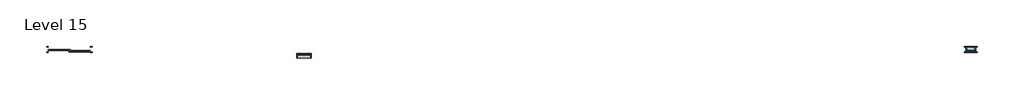
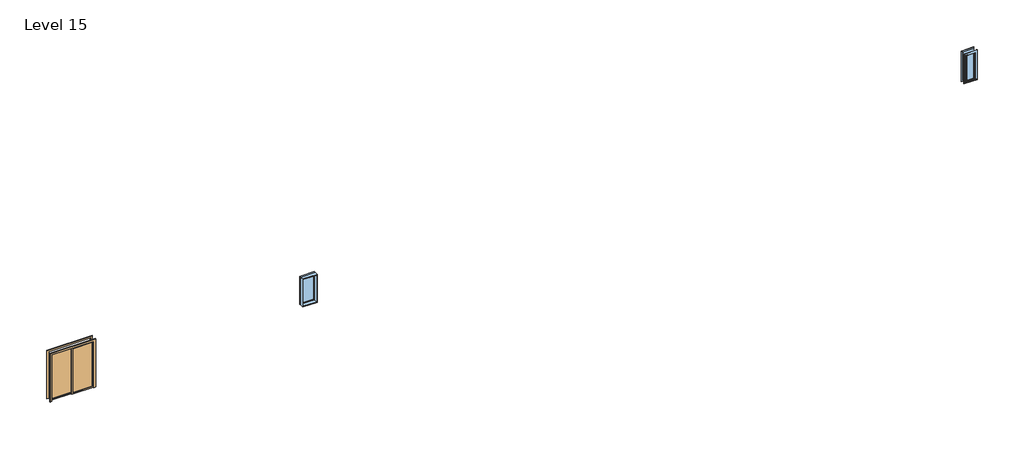
# One storey: 2 windows, 1 door.
"""IFC4 building model written with IfcOpenShell, lengths in millimetres."""

from ifc_helpers import new_model, si_unit, origin, place, context, project, spatial, transform, mapped, element, save
from components import door_076b30e0, window_a765b88f, window_80bd9af0

model = new_model("IFC4")

# Units and contexts
model_context = context("Model", 3, world=origin())
ifc_project = project(units=[si_unit("LENGTHUNIT", "METRE", prefix="MILLI")], contexts=[model_context])

# Site, building, storey
site = spatial("IfcSite", under=ifc_project)
building = spatial("IfcBuilding", under=site)
storey = spatial("IfcBuildingStorey", under=building, Name="Level 15", Elevation=26212.8)

# Door
placement = place(None, origin())
door_shape = door_076b30e0(model_context)
element("IfcDoor", 1, ObjectType="Door-Double-Sliding : 68\" x 80\"", at=placement, inside=storey, context=model_context, shape_type="MappedRepresentation", body=[
    mapped(door_shape, transform((-16115.385279, -12227.7237084, 26430.5574534), x_axis=(-1.0, 0.0, 0.0), y_axis=(0.0, -1.0, 0.0), z_axis=(0.0, 0.0, 1.0))),
])

# Windows
window_shape = window_a765b88f(model_context)
element("IfcWindow", 2, ObjectType="Awning with Trim : 16\" x 48\"", at=placement, inside=storey, context=model_context, shape_type="MappedRepresentation", body=[
    mapped(window_shape, transform((20968.614721, -12354.7237084, 26212.8), x_axis=(-1.0, 0.0, 0.0), y_axis=(0.0, -1.0, 0.0), z_axis=(0.0, 0.0, 1.0))),
])
window_2_shape = window_80bd9af0(model_context)
element("IfcWindow", 3, ObjectType="Fixed : 24\" x 48\"", at=placement, inside=storey, context=model_context, shape_type="MappedRepresentation", body=[
    mapped(window_2_shape, transform((-6425.285279, -12617.2007309, 26212.8), x_axis=(1.0, 0.0, 0.0), y_axis=(0.0, 1.0, 0.0), z_axis=(0.0, 0.0, 1.0))),
])

save(model, "model.ifc")

# Revit data of these elements
# Type "Door-Double-Sliding : 68\" x 80\""
#   Type Mark = "10"
#   Construction Type Id = "opn-d45"
#   Assembly Code = "C1020"
#   Analytic Construction = "Wood frame, double glass door "
#   Thickness = 0' - 2"
#   Thermal Resistance (R) = 1.8150 (h·ft²·°F)/BTU
#   Heat Transfer Coefficient (U) = 0.5510 BTU/(h·ft²·°F)
#   Height = 6' - 8"
#   Rail Width = 0' - 2"
#   Stiles = 0' - 2"
#   Trim Projection Ext = 0' - 1"
#   Trim Projection Int = 0' - 1"
#   Trim Width = 0' - 3"
#   Width = 5' - 8"
#   Define Thermal Properties by = 1
#   Glazing = Glass
#   Panel Material = Wood - Birch - Solid Stained Light Low Gloss
#   Trim Material = Paint - Sienna
#   Visual Light Transmittance = 0
#   Solar Heat Gain Coefficient = 0
#   Function = (empty or 0)
#   Wall Closure = (empty or 0)
# Type "Awning with Trim : 16\" x 48\""
#   Type Mark = "14"
#   Construction Type Id = "GSP4R"
#   Assembly Code = "B2020100"
#   Analytic Construction = "1/8 in Pilkington single glazing"
#   Visual Light Transmittance = 0.9
#   Solar Heat Gain Coefficient = 0.78
#   Heat Transfer Coefficient (U) = 0.6496 BTU/(h·ft²·°F)
#   Height = 4' - 0"
#   Default Sill Height = 3' - 0"
#   Trim Projection - Ext. = 0' - 0 1/2"
#   Trim Projection - Int. = 0' - 0 3/4"
#   Trim Width - Exterior = 0' - 3 1/2"
#   Trim Width - Interior = 0' - 3 1/2"
#   Width = 1' - 4"
#   Window Inset = 0' - 0 3/4"
#   Define Thermal Properties by = 1
#   Glass Pane Material = Glass
#   Sash Material = Sash
#   Trim Exterior Material = Trim
#   Trim Interior Material = Trim
#   Wall Closure = (empty or 0)
# Type "Fixed : 24\" x 48\""
#   Type Mark = "2"
#   Construction Type Id = "GSP4R"
#   Assembly Code = "B2020100"
#   Analytic Construction = "1/8 in Pilkington single glazing"
#   Visual Light Transmittance = 0.9
#   Solar Heat Gain Coefficient = 0.78
#   Heat Transfer Coefficient (U) = 0.6496 BTU/(h·ft²·°F)
#   Height = 4' - 0"
#   Default Sill Height = 3' - 0"
#   Width = 2' - 0"
#   Window Inset = 0' - 0 3/4"
#   Define Thermal Properties by = 1
#   Glass Pane Material = Glass
#   Sash Material = Sash
#   Wall Closure = (empty or 0)
# Element 1 (IfcDoor, "Door-Double-Sliding : 68\" x 80\"")
#   Phase Created = New Construction
#   Materials on its faces: "Paint - Sienna", "Wood - Birch - Solid Stained Light Low Gloss", "Glass"
# Element 2 (IfcWindow, "Awning with Trim : 16\" x 48\"")
#   Mark = "60"
#   Phase Created = New Construction
#   Materials on its faces: "Sash", "Trim", "Glass"
# Element 3 (IfcWindow, "Fixed : 24\" x 48\"")
#   Mark = "77"
#   Phase Created = New Construction
#   Materials on its faces: "Sash", "Glass"
# Materials
#   "Glass": class "Glass", colour RGB 0 128 192, transparency 0.75, Description = "Soda Lime Glass", Cost = 0
#   "Wood - Birch - Solid Stained Light Low Gloss": class "Wood", colour RGB 210 159 95, transparency 0, Cost = 0
#   "Paint - Sienna": colour RGB 118 70 51, transparency 0, Cost = 0
#   "Sash": class "Wood", colour RGB 224 178 126, transparency 0
#   "Trim": class "Wood", colour RGB 224 178 126, transparency 0
